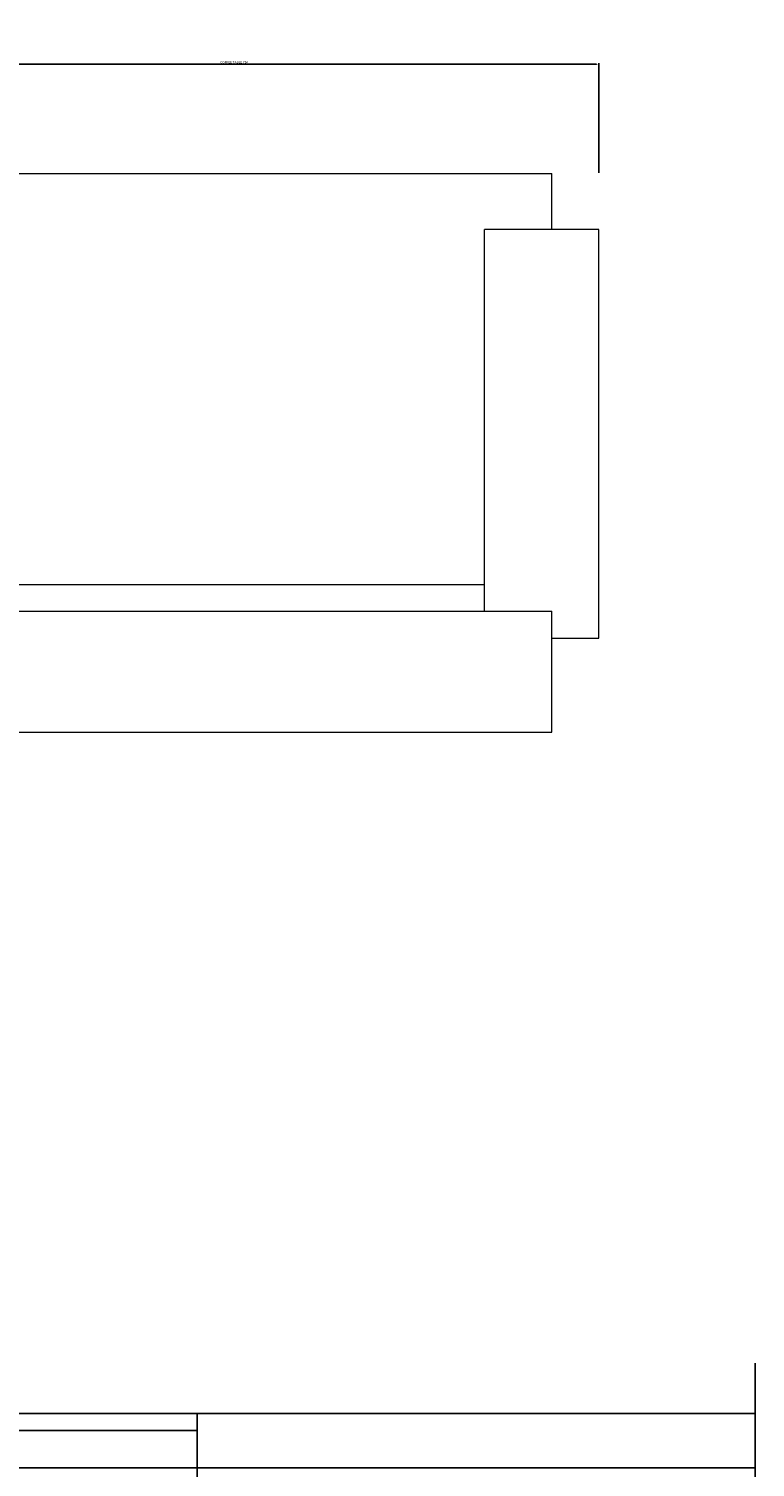
# Model space of a CAD drawing. Units: millimetres. Extents: x -857 to 54106, y -13666 to 13947.
# Tile 8 of 41: x 8305 to 9086, y 5442 to 6990. Entities that reach past the tile are written whole.
import ezdxf

# ---------------------------------------------------------------- set-up
doc = ezdxf.new("R2010")
doc.units = ezdxf.units.MM
for name, color, linetype, lineweight in [('A-ANNO-DIMS', 2, 'Continuous', 18), ('A-FLOR-PATT', 252, 'Continuous', 13), ('A-FURN', 21, 'Continuous', 18), ('A-FURNITURE', 25, 'Continuous', 9), ('A-GLAZ', 4, 'Continuous', 25)]:
    doc.layers.add(name, color=color, linetype=linetype, lineweight=lineweight)
doc.styles.get("Standard").update_dxf_attribs({"font": 'arial.ttf'})
doc.dimstyles.new('ISO-25', dxfattribs={"dimtxt": 2.5, "dimasz": 2.5, "dimexe": 1.25, "dimexo": 0.625, "dimtad": 1, "dimtxsty": 'Standard', "dimcen": 2.5, "dimadec": 0, "dimazin": 0, "dimtfac": 1, "dimtmove": 0, "dimatfit": 3, "dimfxl": 1, "dimarcsym": 0})

# ---------------------------------------------------------------- blocks, each defined once
blk = doc.blocks.new('A$C47E27A62')
at = {"layer": 'A-FURNITURE'}
for p, q in [((17.041, 0), (-17.041, 0)), ((-17.041, 0), (-17.041, -6.486)), ((17.041, 0), (17.041, -6.486)), ((-17.041, -5.045), (-19.563, -5.045)), ((-19.563, -5.045), (-19.563, -26.997)), ((17.041, -5.045), (19.563, -5.045)), ((19.563, -5.045), (19.563, -26.997)), ((17.041, -6.486), (-17.041, -6.486)), ((-13.437, -6.486), (-13.437, -7.927)), ((13.437, -6.486), (13.437, -26.997)), ((13.437, -7.927), (-13.437, -7.927)), ((-13.437, -7.927), (-13.437, -26.997)), ((-19.563, -26.997), (-13.437, -26.997)), ((-17.041, -26.997), (-17.041, -30)), ((19.563, -26.997), (13.437, -26.997)), ((17.041, -26.997), (17.041, -30)), ((17.041, -30), (-17.041, -30))]:
    blk.add_line(p, q, dxfattribs=at)
blk = doc.blocks.new('WIN-1200')
for p, q in [((9371.3, 11750.2), (10571.3, 11750.2)), ((9971.3, 11750.2), (9971.3, 11630.7)), ((9371.3, 11731.7), (9971.3, 11731.7)), ((9371.3, 11691.7), (10571.3, 11691.7)), ((9971.3, 11651.7), (10571.3, 11651.7)), ((10571.3, 11630.7), (9371.3, 11630.7))]:
    blk.add_line(p, q)
for points in [[(9371.3, 11579.2), (9371.3, 11804.2)], [(10571.3, 11804.2), (10571.3, 11579.2)]]:
    blk.add_lwpolyline(points)
blk = doc.blocks.new('*D59')
at = {"layer": 'A-ANNO-DIMS', "color": 0, "lineweight": -2, "transparency": 16777216}
for p, q in [((8134.2, 6835), (8134.2, 6953.2)), ((8915.6, 6952), (8136.7, 6952)), ((8918.1, 6835), (8918.1, 6953.2))]:
    blk.add_line(p, q, dxfattribs=at)
at = {"layer": 'A-ANNO-DIMS', "color": 0, "transparency": 16777216}
for points in [[(8136.7, 6952.4), (8136.7, 6951.6), (8134.2, 6952)], [(8915.6, 6952.4), (8915.6, 6951.6), (8918.1, 6952)]]:
    blk.add_solid(points, dxfattribs=at)
at = {"layer": 'Defpoints', "color": 0, "transparency": 16777216}
for p in [(8134.2, 6952), (8134.2, 6834.4), (8918.1, 6834.4)]:
    blk.add_point(p, dxfattribs=at)
at = {"layer": 'A-ANNO-DIMS', "color": 0, "transparency": 16777216, "insert": (8526.2, 6953.9), "char_height": 2.5, "attachment_point": 5}
blk.add_mtext('COFFEE TABLE 784', dxfattribs=at)

msp = doc.modelspace()

# ---------------------------------------------------------------- hatches: boundary and pattern name
at = {"layer": 'A-FLOR-PATT'}
h = msp.add_hatch(dxfattribs=at)
h.set_pattern_fill('CROSS', color=256, scale=50)
h.set_pattern_definition([(0, (-5489.92, -2561.3), (317.5, 317.5), [158.75, -476.25]), (90, (-5410.54, -2640.7), (-317.5, 317.5), [158.75, -476.25])])
h.paths.add_polyline_path([(16392.264, 9351.555), (14441.85, 9351.555), (13967.28, 9353.369), (13967.28, 9241.901), (13967.28, 8421.901), (13967.28, 6326.555), (16392.264, 6326.555)])
h.paths.add_polyline_path([(16392.264, 12804.231), (14667.264, 12804.231), (14667.264, 12374.147, -0.32131534), (15142.28, 11711.288), (14667.264, 11711.288), (14667.264, 11601.555), (16392.264, 11601.555)])
h.paths.add_polyline_path([(11417.28, 12804.231), (8617.28, 12804.231), (8617.28, 11804.231), (9371.341, 11804.231), (9371.341, 11750.152), (10571.341, 11750.152), (10571.341, 11804.231), (11417.28, 11804.231)])

# ---------------------------------------------------------------- block references
at = {"layer": 'A-FURN', "ltscale": 4, "xscale": 20.03650789584363, "yscale": 20.03650789584363, "zscale": 20.03650789584363, "rotation": 180}
msp.add_blockref('A$C47E27A62', (8526.165, 6233.305), dxfattribs=at)
at = {"layer": 'A-GLAZ'}
msp.add_blockref('WIN-1200', (-1485.087, -6250), dxfattribs=at)

# ---------------------------------------------------------------- dimensions: what is measured, and where the dimension line sits
at = {"layer": 'A-ANNO-DIMS'}
dim = msp.add_linear_dim(base=(8134.194, 6951.992), p1=(8918.137, 6834.4), p2=(8134.194, 6834.4), angle=180, text='COFFEE TABLE <>', dimstyle='ISO-25', override={"dimdec": 0, "dimrnd": 0, "dimzin": 0, "dimlunit": 2}, dxfattribs=at)
dim.commit()
dim.dimension.update_dxf_attribs({"geometry": '*D59', "text_midpoint": (8526.165, 6953.91)})

doc.saveas('drawing.dxf')
